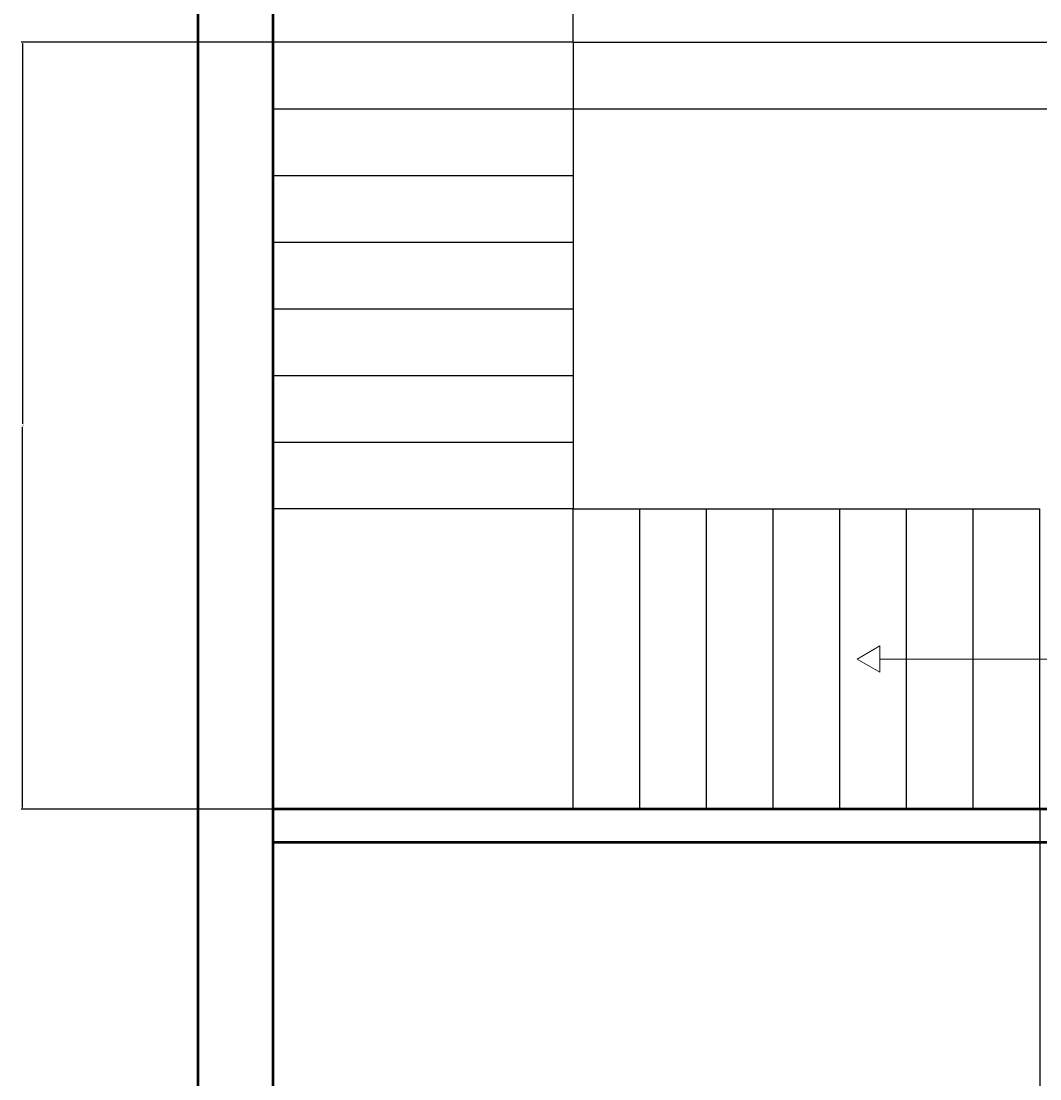
# Model space of a CAD drawing. Units: inches. Extents: x 1798 to 2141, y 1923 to 2386.
# Tile 2 of 9: x 1798 to 1921, y 2050 to 2177. Entities that reach past the tile are written whole.
import ezdxf

# ---------------------------------------------------------------- set-up
doc = ezdxf.new("R2010")
doc.units = ezdxf.units.IN
for name, color, linetype, lineweight in [('A-ANNO-DIMS', 2, 'Continuous', 18), ('A-ANNO-SYMB', 7, 'Continuous', 18), ('A-FLOR-STRS', 3, 'Continuous', 25), ('wall', 4, 'Continuous', 50)]:
    doc.layers.add(name, color=color, linetype=linetype, lineweight=lineweight)
doc.styles.get("Standard").update_dxf_attribs({"font": 'arial.ttf'})
doc.dimstyles.get("Standard").update_dxf_attribs({"dimtxt": 0.18, "dimasz": 0.18, "dimexe": 0.18, "dimexo": 0.0625, "dimgap": 0.09, "dimtad": 0, "dimtih": 1, "dimtoh": 1, "dimdec": 4, "dimzin": 0, "dimdsep": 46, "dimtxsty": 'Standard', "dimcen": 0.09, "dimadec": 0, "dimazin": 0, "dimtfac": 1, "dimtdec": 4, "dimtofl": 0, "dimtmove": 0, "dimatfit": 3, "dimfxl": 1, "dimtolj": 1, "dimtzin": 0, "dimarcsym": 0})

# ---------------------------------------------------------------- blocks, each defined once
blk = doc.blocks.new('*D41')
at = {"layer": 'A-ANNO-DIMS', "color": 0, "lineweight": -2, "transparency": 16777216}
for p, q in [((1828.51, 2082.26), (1828.51, 1923.12)), ((1920.51, 2082.26), (1920.51, 1923.12)), ((1828.69, 1923.3), (1874.3, 1923.3)), ((1920.33, 1923.3), (1874.73, 1923.3))]:
    blk.add_line(p, q, dxfattribs=at)
at = {"layer": 'A-ANNO-DIMS', "color": 0, "transparency": 16777216}
for points in [[(1828.69, 1923.33), (1828.69, 1923.27), (1828.51, 1923.3)], [(1920.33, 1923.33), (1920.33, 1923.27), (1920.51, 1923.3)]]:
    blk.add_solid(points, dxfattribs=at)
at = {"layer": 'Defpoints', "color": 0, "transparency": 16777216}
for p in [(1828.51, 2082.32), (1920.51, 2082.32), (1920.51, 1923.3)]:
    blk.add_point(p, dxfattribs=at)
at = {"layer": 'A-ANNO-DIMS', "color": 0, "transparency": 16777216, "insert": (1874.51, 1923.3), "char_height": 0.18, "attachment_point": 5}
blk.add_mtext('\\A1;92', dxfattribs=at)
blk = doc.blocks.new('*D42')
at = {"layer": 'A-ANNO-DIMS', "color": 0, "lineweight": -2, "transparency": 16777216}
for p, q in [((1828.45, 2174.32), (1798.31, 2174.32)), ((1798.49, 2174.14), (1798.49, 2128.51)), ((1798.49, 2082.5), (1798.49, 2128.14)), ((1828.45, 2082.32), (1798.31, 2082.32))]:
    blk.add_line(p, q, dxfattribs=at)
at = {"layer": 'A-ANNO-DIMS', "color": 0, "transparency": 16777216}
for points in [[(1798.46, 2174.14), (1798.52, 2174.14), (1798.49, 2174.32)], [(1798.46, 2082.5), (1798.52, 2082.5), (1798.49, 2082.32)]]:
    blk.add_solid(points, dxfattribs=at)
at = {"layer": 'Defpoints', "color": 0, "transparency": 16777216}
for p in [(1798.49, 2174.32), (1828.51, 2174.32), (1828.51, 2082.32)]:
    blk.add_point(p, dxfattribs=at)
at = {"layer": 'A-ANNO-DIMS', "color": 0, "transparency": 16777216, "insert": (1798.49, 2128.32), "char_height": 0.18, "attachment_point": 5}
blk.add_mtext('\\A1;92', dxfattribs=at)
blk = doc.blocks.new('*D43')
at = {"layer": 'A-ANNO-DIMS', "color": 0, "lineweight": -2, "transparency": 16777216}
for p, q in [((1828.51, 2174.39), (1828.51, 2385.53)), ((1828.69, 2385.35), (1846.3, 2385.35)), ((1864.33, 2385.35), (1846.73, 2385.35)), ((1864.51, 2174.39), (1864.51, 2385.53))]:
    blk.add_line(p, q, dxfattribs=at)
at = {"layer": 'A-ANNO-DIMS', "color": 0, "transparency": 16777216}
for points in [[(1828.69, 2385.38), (1828.69, 2385.32), (1828.51, 2385.35)], [(1864.33, 2385.38), (1864.33, 2385.32), (1864.51, 2385.35)]]:
    blk.add_solid(points, dxfattribs=at)
at = {"layer": 'Defpoints', "color": 0, "transparency": 16777216}
for p in [(1864.51, 2385.35), (1828.51, 2174.32), (1864.51, 2174.32)]:
    blk.add_point(p, dxfattribs=at)
at = {"layer": 'A-ANNO-DIMS', "color": 0, "transparency": 16777216, "insert": (1846.51, 2385.35), "char_height": 0.18, "attachment_point": 5}
blk.add_mtext('\\A1;36', dxfattribs=at)
blk = doc.blocks.new('*D45')
at = {"layer": 'A-ANNO-DIMS', "color": 0, "lineweight": -2, "transparency": 16777216}
for p, q in [((1864.58, 2174.32), (2140.72, 2174.32)), ((2140.54, 2174.14), (2140.54, 2170.51)), ((2140.54, 2166.5), (2140.54, 2170.14)), ((1864.58, 2166.32), (2140.72, 2166.32))]:
    blk.add_line(p, q, dxfattribs=at)
at = {"layer": 'A-ANNO-DIMS', "color": 0, "transparency": 16777216}
for points in [[(2140.51, 2174.14), (2140.57, 2174.14), (2140.54, 2174.32)], [(2140.51, 2166.5), (2140.57, 2166.5), (2140.54, 2166.32)]]:
    blk.add_solid(points, dxfattribs=at)
at = {"layer": 'Defpoints', "color": 0, "transparency": 16777216}
for p in [(1864.51, 2174.32), (2140.54, 2174.32), (1864.51, 2166.32)]:
    blk.add_point(p, dxfattribs=at)
at = {"layer": 'A-ANNO-DIMS', "color": 0, "transparency": 16777216, "insert": (2140.54, 2170.32), "char_height": 0.18, "attachment_point": 5}
blk.add_mtext('\\A1;8', dxfattribs=at)

msp = doc.modelspace()

# ---------------------------------------------------------------- linework, layer by layer
at = {"layer": 'A-ANNO-SYMB'}
msp.add_line((1932.1142, 2100.3239), (1901.337, 2100.3239), dxfattribs=at)
msp.add_lwpolyline([(1901.337, 2098.7353), (1901.337, 2101.9125), (1898.5854, 2100.3239)], close=True, dxfattribs=at)
at = {"layer": 'A-FLOR-STRS'}
for p, q in [((1828.5141, 2174.3239), (1864.5141, 2174.3239)), ((1828.5141, 2174.3239), (1828.5141, 2166.3239)), ((1864.5141, 2174.3239), (1864.5141, 2166.3239)), ((1828.5141, 2166.3239), (1864.5141, 2166.3239)), ((1828.5141, 2166.3239), (1828.5141, 2158.3239)), ((1864.5141, 2166.3239), (1864.5141, 2158.3239)), ((1828.5141, 2158.3239), (1864.5141, 2158.3239)), ((1828.5141, 2158.3239), (1828.5141, 2150.3239)), ((1864.5141, 2158.3239), (1864.5141, 2150.3239)), ((1828.5141, 2150.3239), (1864.5141, 2150.3239)), ((1864.5141, 2150.3239), (1864.5141, 2142.3239)), ((1828.5141, 2142.3239), (1864.5141, 2142.3239)), ((1828.5141, 2142.3239), (1828.5141, 2134.3239)), ((1864.5141, 2142.3239), (1864.5141, 2134.3239)), ((1828.5141, 2134.3239), (1864.5141, 2134.3239)), ((1828.5141, 2134.3239), (1828.5141, 2126.3239)), ((1864.5141, 2134.3239), (1864.5141, 2126.3239)), ((1828.5141, 2126.3239), (1864.5141, 2126.3239)), ((1828.5141, 2126.3239), (1828.5141, 2118.3239)), ((1864.5141, 2126.3239), (1864.5141, 2118.3239)), ((1864.5141, 2118.3239), (1828.5141, 2118.3239)), ((1828.5141, 2118.3239), (1828.5141, 2082.3239)), ((1864.5141, 2082.3239), (1864.5141, 2118.3239)), ((1864.5141, 2118.3239), (1872.5141, 2118.3239)), ((1872.5141, 2082.3239), (1872.5141, 2118.3239)), ((1872.5141, 2118.3239), (1880.5141, 2118.3239)), ((1880.5141, 2082.3239), (1880.5141, 2118.3239)), ((1880.5141, 2118.3239), (1888.5141, 2118.3239)), ((1888.5141, 2082.3239), (1888.5141, 2118.3239)), ((1888.5141, 2118.3239), (1896.5141, 2118.3239)), ((1896.5141, 2082.3239), (1896.5141, 2118.3239)), ((1896.5141, 2118.3239), (1904.5141, 2118.3239)), ((1904.5141, 2082.3239), (1904.5141, 2118.3239)), ((1904.5141, 2118.3239), (1912.5141, 2118.3239)), ((1912.5141, 2082.3239), (1912.5141, 2118.3239)), ((1912.5141, 2118.3239), (1920.5141, 2118.3239)), ((1920.5141, 2082.3239), (1920.5141, 2118.3239)), ((1828.5141, 2082.3239), (1864.5141, 2082.3239)), ((1864.5141, 2082.3239), (1872.5141, 2082.3239)), ((1872.5141, 2082.3239), (1880.5141, 2082.3239)), ((1880.5141, 2082.3239), (1888.5141, 2082.3239)), ((1888.5141, 2082.3239), (1896.5141, 2082.3239)), ((1896.5141, 2082.3239), (1904.5141, 2082.3239)), ((1904.5141, 2082.3239), (1912.5141, 2082.3239)), ((1912.5141, 2082.3239), (1920.5141, 2082.3239))]:
    msp.add_line(p, q, dxfattribs=at)
msp.add_lwpolyline([(1864.5141, 2082.3239), (1864.5141, 2082.3239), (1864.5141, 2082.3239), (1864.5141, 2082.3239)], close=True, dxfattribs=at)
at = {"layer": 'wall'}
for p, q in [((1819.5141, 2364.3239), (1819.5141, 1944.3239)), ((1828.5141, 2355.3239), (1828.5141, 1953.3239)), ((1976.5141, 2082.3239), (1828.5141, 2082.3239)), ((1972.5141, 2078.3239), (1828.5141, 2078.3239))]:
    msp.add_line(p, q, dxfattribs=at)

# ---------------------------------------------------------------- dimensions: what is measured, and where the dimension line sits
at = {"layer": 'A-ANNO-DIMS'}
for base, p1, p2, picture, middle in [((1864.5141, 2385.3489), (1828.5141, 2174.3239), (1864.5141, 2174.3239), '*D43', (1846.5141, 2385.3489)), ((1920.5141, 1923.2989), (1828.5141, 2082.3239), (1920.5141, 2082.3239), '*D41', (1874.5141, 1923.2989))]:
    dim = msp.add_linear_dim(base=base, p1=p1, p2=p2, dimstyle='Standard', override={"dimdec": 0, "dimlfac": 1, "dimrnd": 0, "dimzin": 0, "dimdsep": 46, "dimlunit": 2}, dxfattribs=at)
    dim.commit()
    dim.dimension.update_dxf_attribs({"geometry": picture, "text_midpoint": middle})
for base, p1, p2, picture, middle in [((1798.4891, 2174.3239), (1828.5141, 2082.3239), (1828.5141, 2174.3239), '*D42', (1798.4891, 2128.3239)), ((2140.5391, 2174.3239), (1864.5141, 2166.3239), (1864.5141, 2174.3239), '*D45', (2140.5391, 2170.3239))]:
    dim = msp.add_linear_dim(base=base, p1=p1, p2=p2, angle=90, dimstyle='Standard', override={"dimdec": 0, "dimlfac": 1, "dimrnd": 0, "dimzin": 0, "dimdsep": 46, "dimlunit": 2}, dxfattribs=at)
    dim.commit()
    dim.dimension.update_dxf_attribs({"geometry": picture, "text_midpoint": middle})

doc.saveas('drawing.dxf')
